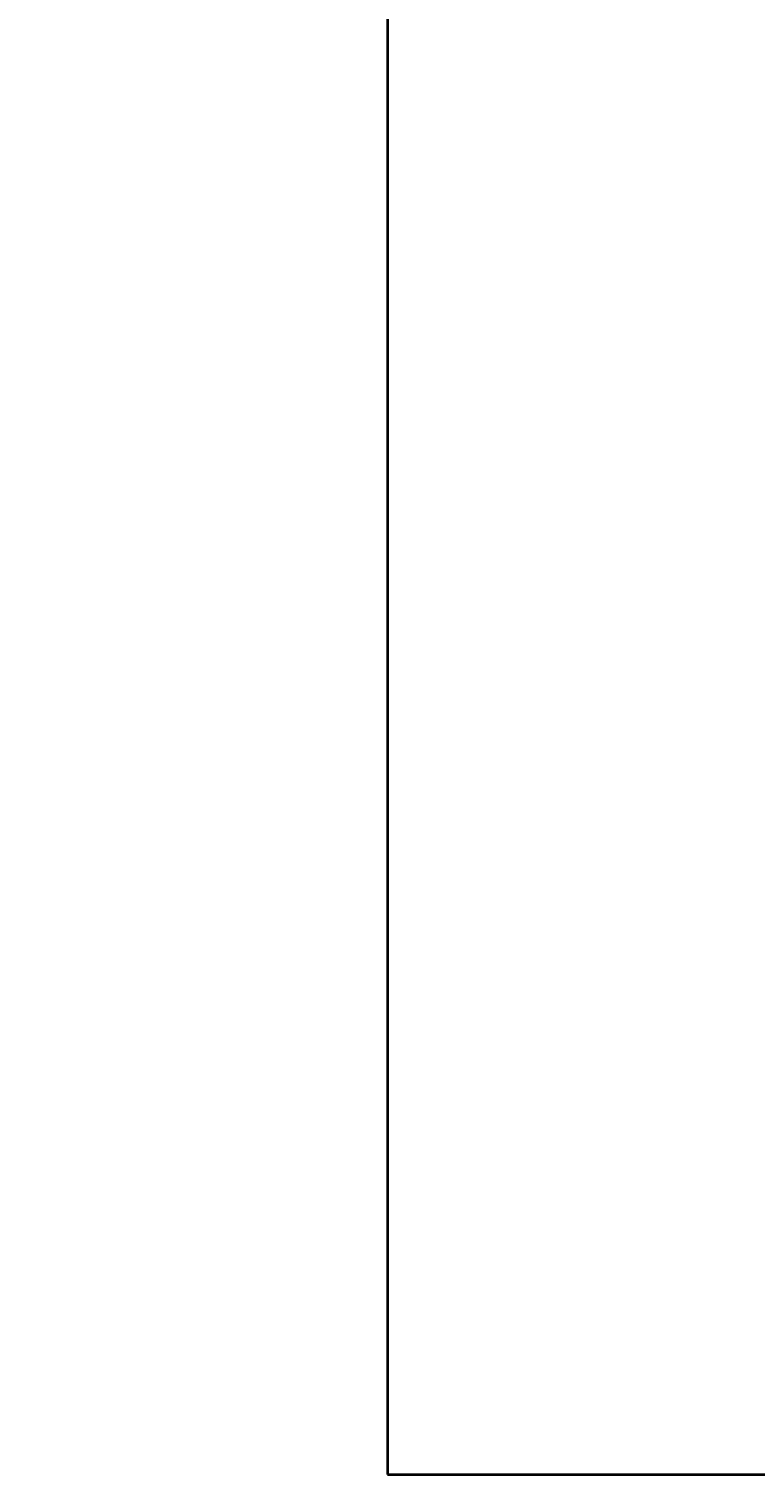
# Model space of a CAD drawing. Units: millimetres. Extents: x 27017497 to 27018854, y 7058029 to 7059154.
# Tile 4 of 91: x 27017605 to 27017622, y 7058133 to 7058166. Entities that reach past the tile are written whole.
import ezdxf

# ---------------------------------------------------------------- set-up
doc = ezdxf.new("R2010")
doc.units = ezdxf.units.MM
doc.layers.add('A-ANNO-DIMS', color=2, linetype='Continuous', lineweight=18)
doc.layers.add('A-WALL', color=7, linetype='Continuous', lineweight=35)
doc.styles.get("Standard").update_dxf_attribs({"font": 'arial.ttf'})
doc.dimstyles.get("Standard").update_dxf_attribs({"dimtxt": 0.18, "dimasz": 0.18, "dimexe": 0.18, "dimexo": 0.0625, "dimgap": 0.09, "dimtad": 0, "dimtih": 1, "dimtoh": 1, "dimdec": 4, "dimzin": 0, "dimdsep": 46, "dimtxsty": 'Standard', "dimcen": 0.09, "dimadec": 0, "dimazin": 0, "dimtfac": 1, "dimtdec": 4, "dimtofl": 0, "dimtmove": 0, "dimatfit": 3, "dimfxl": 1, "dimtolj": 1, "dimtzin": 0, "dimarcsym": 0})

# ---------------------------------------------------------------- blocks, each defined once
blk = doc.blocks.new('*D47')
at = {"layer": 'A-ANNO-DIMS', "color": 0, "lineweight": -2, "transparency": 16777216}
for p, q in [((27017561.166, 7058294.35), (27017561.166, 7058028.6)), ((27018790.606, 7058294.35), (27018790.606, 7058028.6)), ((27017561.346, 7058028.78), (27018175.431, 7058028.78)), ((27018790.426, 7058028.78), (27018176.341, 7058028.78))]:
    blk.add_line(p, q, dxfattribs=at)
at = {"layer": 'A-ANNO-DIMS', "color": 0, "transparency": 16777216}
for points in [[(27017561.346, 7058028.81), (27017561.346, 7058028.75), (27017561.166, 7058028.78)], [(27018790.426, 7058028.81), (27018790.426, 7058028.75), (27018790.606, 7058028.78)]]:
    blk.add_solid(points, dxfattribs=at)
at = {"layer": 'Defpoints', "color": 0, "transparency": 16777216}
for p in [(27017561.166, 7058294.412), (27018790.606, 7058294.412), (27018790.606, 7058028.78)]:
    blk.add_point(p, dxfattribs=at)
at = {"layer": 'A-ANNO-DIMS', "color": 0, "transparency": 16777216, "insert": (27018175.886, 7058028.78), "char_height": 0.18, "attachment_point": 5}
blk.add_mtext('\\A1;1229.4', dxfattribs=at)
blk = doc.blocks.new('*D48')
at = {"layer": 'A-ANNO-DIMS', "color": 0, "lineweight": -2, "transparency": 16777216}
for p, q in [((27018463.498, 7058622.912), (27017497.536, 7058622.912)), ((27017497.716, 7058622.732), (27017497.716, 7058357.753)), ((27017497.716, 7058092.41), (27017497.716, 7058357.389)), ((27018555.129, 7058092.23), (27017497.536, 7058092.23))]:
    blk.add_line(p, q, dxfattribs=at)
at = {"layer": 'A-ANNO-DIMS', "color": 0, "transparency": 16777216}
for points in [[(27017497.686, 7058622.732), (27017497.746, 7058622.732), (27017497.716, 7058622.912)], [(27017497.686, 7058092.41), (27017497.746, 7058092.41), (27017497.716, 7058092.23)]]:
    blk.add_solid(points, dxfattribs=at)
at = {"layer": 'Defpoints', "color": 0, "transparency": 16777216}
for p in [(27018463.561, 7058622.912), (27017497.716, 7058092.23), (27018555.192, 7058092.23)]:
    blk.add_point(p, dxfattribs=at)
at = {"layer": 'A-ANNO-DIMS', "color": 0, "transparency": 16777216, "insert": (27017497.716, 7058357.571), "char_height": 0.18, "attachment_point": 5}
blk.add_mtext('\\A1;530.7', dxfattribs=at)

msp = doc.modelspace()

# ---------------------------------------------------------------- linework, layer by layer
at = {"layer": 'A-WALL'}
for p, q in [((27017613.666, 7058294.412), (27017613.666, 7058132.912)), ((27017613.666, 7058132.912), (27017802.166, 7058132.912)), ((27017613.666, 7058132.912), (27017802.166, 7058132.912))]:
    msp.add_line(p, q, dxfattribs=at)

# ---------------------------------------------------------------- dimensions: what is measured, and where the dimension line sits
at = {"layer": 'A-ANNO-DIMS'}
dim = msp.add_linear_dim(base=(27017497.716, 7058092.23), p1=(27018463.561, 7058622.912), p2=(27018555.192, 7058092.23), angle=90, dimstyle='Standard', override={"dimdec": 1, "dimlfac": 1, "dimrnd": 0, "dimzin": 0, "dimdsep": 46, "dimlunit": 2}, dxfattribs=at)
dim.commit()
dim.dimension.update_dxf_attribs({"geometry": '*D48', "text_midpoint": (27017497.716, 7058357.571)})
dim = msp.add_linear_dim(base=(27018790.606, 7058028.78), p1=(27017561.166, 7058294.412), p2=(27018790.606, 7058294.412), dimstyle='Standard', override={"dimdec": 1, "dimlfac": 1, "dimrnd": 0, "dimzin": 0, "dimdsep": 46, "dimlunit": 2}, dxfattribs=at)
dim.commit()
dim.dimension.update_dxf_attribs({"geometry": '*D47', "text_midpoint": (27018175.886, 7058028.78)})

doc.saveas('drawing.dxf')
